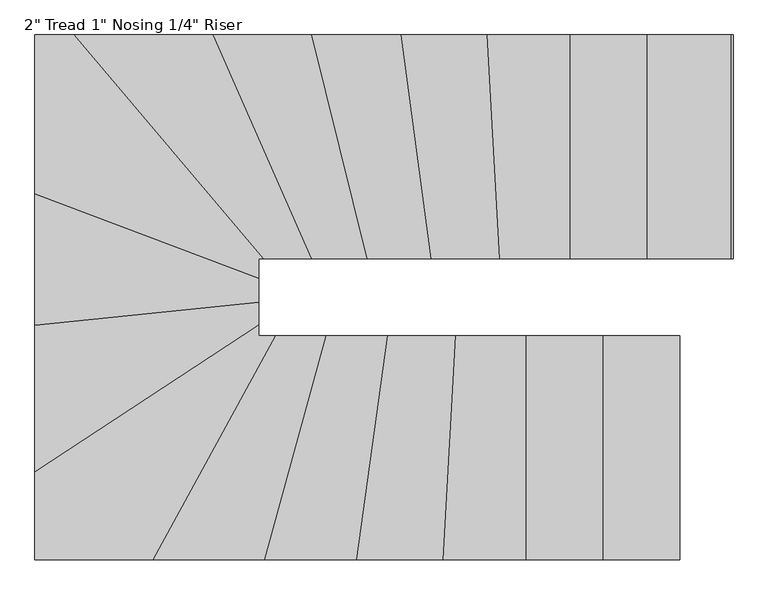
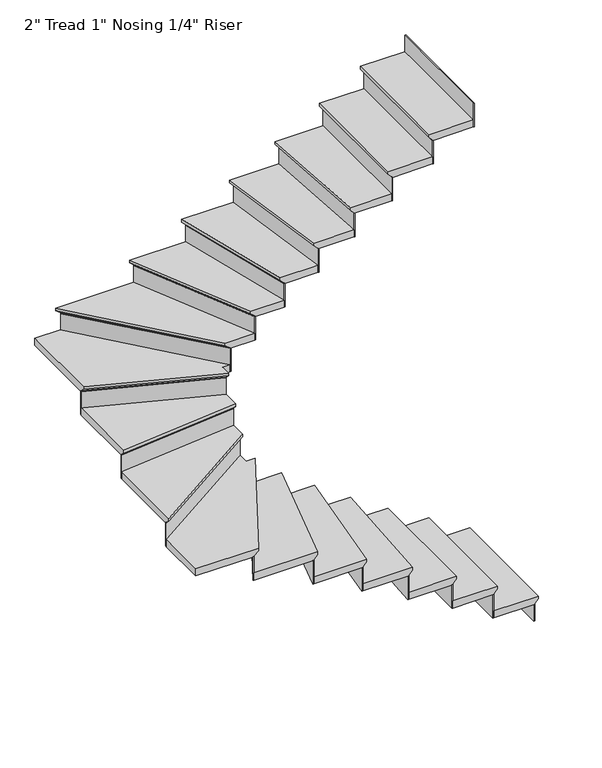
"""IFC4 building model written with IfcOpenShell, lengths in millimetres: stair flight geometry."""

from ifc_helpers import new_model, si_unit, origin, place, context, project, spatial, faceted_brep, source, transform, mapped, element, save


def stair_flight_2a3e21a6(model_context):
    return source(origin(), model_context, "Body", "Brep", [
        faceted_brep([(-12253.9414615, 8989.1162111, 150.2833333), (-12253.9414615, 8989.1162111, 169.3333333), (-12253.9414615, 8176.3162111, 169.3333333), (-12253.9414615, 8176.3162111, 150.2833333), (-12279.3414615, 8989.1162111, 124.8833333), (-12279.3414615, 8176.3162111, 124.8833333), (-12558.7414615, 8989.1162111, 169.3333333), (-12558.7414615, 8176.3162111, 169.3333333), (-12279.3414615, 8176.3162111, 118.5333333), (-12558.7414615, 8176.3162111, 118.5333333), (-12558.7414615, 8989.1162111, 118.5333333), (-12279.3414615, 8989.1162111, 118.5333333)], [[[0, 1, 2, 3]], [[4, 0, 3, 5]], [[2, 1, 6, 7]], [[8, 9, 10, 11]], [[2, 7, 9, 8, 5, 3]], [[8, 11, 4, 5]], [[6, 1, 0, 4, 11, 10]], [[7, 6, 10, 9]]]),
        faceted_brep([(-12279.3414615, 8989.1162111, 118.5333333), (-12279.3414615, 8989.1162111, 0.0), (-12285.6914615, 8989.1162111, 0.0), (-12285.6914615, 8989.1162111, 118.5333333), (-12279.3414615, 8176.3162111, 118.5333333), (-12285.6914615, 8176.3162111, 118.5333333), (-12285.6914615, 8176.3162111, 0.0), (-12279.3414615, 8176.3162111, 0.0)], [[[0, 1, 2, 3]], [[4, 5, 6, 7]], [[1, 0, 4, 7]], [[2, 1, 7, 6]], [[3, 2, 6, 5]], [[0, 3, 5, 4]]]),
        faceted_brep([(-12558.7414615, 8989.1162111, 287.8666667), (-12558.7414615, 8989.1162111, 118.5333333), (-12565.0914615, 8989.1162111, 118.5333333), (-12565.0914615, 8989.1162111, 287.8666667), (-12558.7414615, 8176.3162111, 287.8666667), (-12565.0914615, 8176.3162111, 287.8666667), (-12565.0914615, 8176.3162111, 118.5333333), (-12558.7414615, 8176.3162111, 118.5333333)], [[[0, 1, 2, 3]], [[4, 5, 6, 7]], [[1, 0, 4, 7]], [[2, 1, 7, 6]], [[3, 2, 6, 5]], [[0, 3, 5, 4]]]),
        faceted_brep([(-12533.3414615, 8176.3162111, 338.6666667), (-12533.3414615, 8989.1162111, 338.6666667), (-12838.1414615, 8989.1162111, 338.6666667), (-12838.1414615, 8176.3162111, 338.6666667), (-12558.7414615, 8176.3162111, 287.8666667), (-12838.1414615, 8176.3162111, 287.8666667), (-12838.1414615, 8989.1162111, 287.8666667), (-12558.7414615, 8989.1162111, 287.8666667), (-12558.7414615, 8176.3162111, 294.2166667), (-12533.3414615, 8176.3162111, 319.6166667), (-12558.7414615, 8989.1162111, 294.2166667), (-12533.3414615, 8989.1162111, 319.6166667)], [[[0, 1, 2, 3]], [[4, 5, 6, 7]], [[0, 3, 5, 4, 8, 9]], [[4, 7, 10, 8]], [[2, 1, 11, 10, 7, 6]], [[3, 2, 6, 5]], [[11, 1, 0, 9]], [[10, 11, 9, 8]]]),
        faceted_brep([(-12838.1414615, 8989.1162111, 457.2), (-12838.1414615, 8989.1162111, 287.8666667), (-12844.4914615, 8989.1162111, 287.8666667), (-12844.4914615, 8989.1162111, 457.2), (-12838.1414615, 8176.3162111, 457.2), (-12844.4914615, 8176.3162111, 457.2), (-12844.4914615, 8176.3162111, 287.8666667), (-12838.1414615, 8176.3162111, 287.8666667)], [[[0, 1, 2, 3]], [[4, 5, 6, 7]], [[1, 0, 4, 7]], [[2, 1, 7, 6]], [[3, 2, 6, 5]], [[0, 3, 5, 4]]]),
        faceted_brep([(-12812.7414615, 8176.3162111, 508.0), (-12812.7414615, 8989.1162111, 508.0), (-13095.0084855, 8989.1162111, 508.0), (-13140.152733, 8176.3162111, 508.0), (-12838.1414615, 8176.3162111, 457.2), (-13140.152733, 8176.3162111, 457.2), (-13095.0084855, 8989.1162111, 457.2), (-12838.1414615, 8989.1162111, 457.2), (-12838.1414615, 8176.3162111, 463.55), (-12812.7414615, 8176.3162111, 488.95), (-12838.1414615, 8989.1162111, 463.55), (-12812.7414615, 8989.1162111, 488.95)], [[[0, 1, 2, 3]], [[4, 5, 6, 7]], [[0, 3, 5, 4, 8, 9]], [[4, 7, 10, 8]], [[2, 1, 11, 10, 7, 6]], [[3, 2, 6, 5]], [[11, 1, 0, 9]], [[10, 11, 9, 8]]]),
        faceted_brep([(-13095.0084855, 8989.1162111, 626.5333333), (-13095.0084855, 8989.1162111, 457.2), (-13101.3682724, 8989.1162111, 457.2), (-13101.3682724, 8989.1162111, 626.5333333), (-13140.152733, 8176.3162111, 626.5333333), (-13146.5125199, 8176.3162111, 626.5333333), (-13146.5125199, 8176.3162111, 457.2), (-13140.152733, 8176.3162111, 457.2)], [[[0, 1, 2, 3]], [[4, 5, 6, 7]], [[1, 0, 4, 7]], [[2, 1, 7, 6]], [[3, 2, 6, 5]], [[0, 3, 5, 4]]]),
        faceted_brep([(-13114.7135853, 8176.3162111, 677.3333333), (-13069.5693378, 8989.1162111, 677.3333333), (-13341.0188921, 8989.1162111, 677.3333333), (-13453.3468485, 8176.3162111, 677.3333333), (-13140.152733, 8176.3162111, 626.5333333), (-13453.3468485, 8176.3162111, 626.5333333), (-13341.0188921, 8989.1162111, 626.5333333), (-13095.0084855, 8989.1162111, 626.5333333), (-13140.152733, 8176.3162111, 632.8833333), (-13114.7135853, 8176.3162111, 658.2833333), (-13095.0084855, 8989.1162111, 632.8833333), (-13069.5693378, 8989.1162111, 658.2833333)], [[[0, 1, 2, 3]], [[4, 5, 6, 7]], [[0, 3, 5, 4, 8, 9]], [[4, 7, 10, 8]], [[2, 1, 11, 10, 7, 6]], [[3, 2, 6, 5]], [[11, 1, 0, 9]], [[10, 11, 9, 8]]]),
        faceted_brep([(-13341.0188921, 8989.1162111, 795.8666667), (-13341.0188921, 8989.1162111, 626.5333333), (-13347.4292443, 8989.1162111, 626.5333333), (-13347.4292443, 8989.1162111, 795.8666667), (-13453.3468485, 8176.3162111, 795.8666667), (-13459.7572007, 8176.3162111, 795.8666667), (-13459.7572007, 8176.3162111, 626.5333333), (-13453.3468485, 8176.3162111, 626.5333333)], [[[0, 1, 2, 3]], [[4, 5, 6, 7]], [[1, 0, 4, 7]], [[2, 1, 7, 6]], [[3, 2, 6, 5]], [[0, 3, 5, 4]]]),
        faceted_brep([(-13427.7054397, 8176.3162111, 846.6666667), (-13315.3774833, 8989.1162111, 846.6666667), (-13565.828015, 8989.1162111, 846.6666667), (-13788.7305586, 8176.3162111, 846.6666667), (-13453.3468485, 8176.3162111, 795.8666667), (-13788.7305586, 8176.3162111, 795.8666667), (-13565.828015, 8989.1162111, 795.8666667), (-13341.0188921, 8989.1162111, 795.8666667), (-13453.3468485, 8176.3162111, 802.2166667), (-13427.7054397, 8176.3162111, 827.6166667), (-13341.0188921, 8989.1162111, 802.2166667), (-13315.3774833, 8989.1162111, 827.6166667)], [[[0, 1, 2, 3]], [[4, 5, 6, 7]], [[0, 3, 5, 4, 8, 9]], [[4, 7, 10, 8]], [[2, 1, 11, 10, 7, 6]], [[3, 2, 6, 5]], [[11, 1, 0, 9]], [[10, 11, 9, 8]]]),
        faceted_brep([(-13565.828015, 8989.1162111, 965.2), (-13565.828015, 8989.1162111, 795.8666667), (-13572.4124713, 8989.1162111, 795.8666667), (-13572.4124713, 8989.1162111, 965.2), (-13788.7305586, 8176.3162111, 965.2), (-13795.3150149, 8176.3162111, 965.2), (-13795.3150149, 8176.3162111, 795.8666667), (-13788.7305586, 8176.3162111, 795.8666667)], [[[0, 1, 2, 3]], [[4, 5, 6, 7]], [[1, 0, 4, 7]], [[2, 1, 7, 6]], [[3, 2, 6, 5]], [[0, 3, 5, 4]]]),
        faceted_brep([(-13762.3927333, 8176.3162111, 1016.0), (-13539.4901897, 8989.1162111, 1016.0), (-13750.8519704, 8989.1162111, 1016.0), (-14195.2006773, 8176.3162111, 1016.0), (-13788.7305586, 8176.3162111, 965.2), (-14195.2006773, 8176.3162111, 965.2), (-13750.8519704, 8989.1162111, 965.2), (-13565.828015, 8989.1162111, 965.2), (-13788.7305586, 8176.3162111, 971.55), (-13762.3927333, 8176.3162111, 996.95), (-13565.828015, 8989.1162111, 971.55), (-13539.4901897, 8989.1162111, 996.95)], [[[0, 1, 2, 3]], [[4, 5, 6, 7]], [[0, 3, 5, 4, 8, 9]], [[4, 7, 10, 8]], [[2, 1, 11, 10, 7, 6]], [[3, 2, 6, 5]], [[11, 1, 0, 9]], [[10, 11, 9, 8]]]),
        faceted_brep([(-13750.8519704, 8989.1162111, 1134.5333333), (-13750.8519704, 8989.1162111, 965.2), (-13758.0889334, 8989.1162111, 965.2), (-13758.0889334, 8989.1162111, 1134.5333333), (-14195.2006773, 8176.3162111, 1134.5333333), (-14202.4376404, 8176.3162111, 1134.5333333), (-14202.4376404, 8176.3162111, 965.2), (-14195.2006773, 8176.3162111, 965.2)], [[[0, 1, 2, 3]], [[4, 5, 6, 7]], [[1, 0, 4, 7]], [[2, 1, 7, 6]], [[3, 2, 6, 5]], [[0, 3, 5, 4]]]),
        faceted_brep([(-14594.4731534, 8526.2265371, 1185.3333333), (-14594.4731534, 8176.3162111, 1185.3333333), (-14166.2528253, 8176.3162111, 1185.3333333), (-13721.9041183, 8989.1162111, 1185.3333333), (-13781.6731534, 8989.1162111, 1185.3333333), (-13781.6731534, 9059.6430441, 1185.3333333), (-14594.4731534, 8176.3162111, 1134.5333333), (-14594.4731534, 8526.2265371, 1134.5333333), (-13781.6731534, 9059.6430441, 1134.5333333), (-13781.6731534, 8989.1162111, 1134.5333333), (-13750.8519704, 8989.1162111, 1134.5333333), (-14195.2006773, 8176.3162111, 1134.5333333), (-14195.2006773, 8176.3162111, 1140.8833333), (-14166.2528253, 8176.3162111, 1166.2833333), (-13750.8519704, 8989.1162111, 1140.8833333), (-13721.9041183, 8989.1162111, 1166.2833333)], [[[0, 1, 2, 3, 4, 5]], [[6, 7, 8, 9, 10, 11]], [[1, 0, 7, 6]], [[2, 1, 6, 11, 12, 13]], [[11, 10, 14, 12]], [[4, 3, 15, 14, 10, 9]], [[5, 4, 9, 8]], [[0, 5, 8, 7]], [[15, 3, 2, 13]], [[14, 15, 13, 12]]]),
        faceted_brep([(-13781.6731534, 9059.6430441, 1303.8666667), (-13781.6731534, 9059.6430441, 1134.5333333), (-13781.6731534, 9067.2383734, 1134.5333333), (-13781.6731534, 9067.2383734, 1303.8666667), (-14594.4731534, 8526.2265371, 1303.8666667), (-14594.4731534, 8533.8218664, 1303.8666667), (-14594.4731534, 8533.8218664, 1134.5333333), (-14594.4731534, 8526.2265371, 1134.5333333)], [[[0, 1, 2, 3]], [[4, 5, 6, 7]], [[1, 0, 4, 7]], [[2, 1, 7, 6]], [[3, 2, 6, 5]], [[0, 3, 5, 4]]]),
        faceted_brep([(-14594.4731534, 8495.8452201, 1354.6666667), (-13781.6731534, 9029.2617271, 1354.6666667), (-13781.6731534, 9137.1899259, 1354.6666667), (-14594.4731534, 9053.7994193, 1354.6666667), (-14594.4731534, 8526.2265371, 1303.8666667), (-14594.4731534, 9053.7994193, 1303.8666667), (-13781.6731534, 9137.1899259, 1303.8666667), (-13781.6731534, 9059.6430441, 1303.8666667), (-14594.4731534, 8526.2265371, 1310.2166667), (-14594.4731534, 8495.8452201, 1335.6166667), (-13781.6731534, 9059.6430441, 1310.2166667), (-13781.6731534, 9029.2617271, 1335.6166667)], [[[0, 1, 2, 3]], [[4, 5, 6, 7]], [[0, 3, 5, 4, 8, 9]], [[4, 7, 10, 8]], [[3, 2, 6, 5]], [[11, 1, 0, 9]], [[10, 11, 9, 8]], [[2, 1, 11, 10, 7, 6]]]),
        faceted_brep([(-13781.6731534, 9137.1899259, 1473.2), (-13781.6731534, 9137.1899259, 1303.8666667), (-13781.6731534, 9143.5732587, 1303.8666667), (-13781.6731534, 9143.5732587, 1473.2), (-14594.4731534, 9053.7994193, 1473.2), (-14594.4731534, 9060.182752, 1473.2), (-14594.4731534, 9060.182752, 1303.8666667), (-14594.4731534, 9053.7994193, 1303.8666667)], [[[0, 1, 2, 3]], [[4, 5, 6, 7]], [[1, 0, 4, 7]], [[2, 1, 7, 6]], [[3, 2, 6, 5]], [[0, 3, 5, 4]]]),
        faceted_brep([(-14594.4731534, 9028.2660883, 1524.0), (-13781.6731534, 9111.6565949, 1524.0), (-13781.6731534, 9225.8746832, 1524.0), (-14594.4731534, 9533.0408462, 1524.0), (-14594.4731534, 9053.7994193, 1473.2), (-14594.4731534, 9533.0408462, 1473.2), (-13781.6731534, 9225.8746832, 1473.2), (-13781.6731534, 9137.1899259, 1473.2), (-14594.4731534, 9053.7994193, 1479.55), (-14594.4731534, 9028.2660883, 1504.95), (-13781.6731534, 9137.1899259, 1479.55), (-13781.6731534, 9111.6565949, 1504.95)], [[[0, 1, 2, 3]], [[4, 5, 6, 7]], [[0, 3, 5, 4, 8, 9]], [[4, 7, 10, 8]], [[2, 1, 11, 10, 7, 6]], [[3, 2, 6, 5]], [[11, 1, 0, 9]], [[10, 11, 9, 8]]]),
        faceted_brep([(-13781.6731534, 9225.8746832, 1642.5333333), (-13781.6731534, 9225.8746832, 1473.2), (-13781.6731534, 9232.662999, 1473.2), (-13781.6731534, 9232.662999, 1642.5333333), (-14594.4731534, 9533.0408462, 1642.5333333), (-14594.4731534, 9539.829162, 1642.5333333), (-14594.4731534, 9539.829162, 1473.2), (-14594.4731534, 9533.0408462, 1473.2)], [[[0, 1, 2, 3]], [[4, 5, 6, 7]], [[1, 0, 4, 7]], [[2, 1, 7, 6]], [[3, 2, 6, 5]], [[0, 3, 5, 4]]]),
        faceted_brep([(-14418.4386981, 10081.3162111, 1693.3333333), (-14594.4731534, 10081.3162111, 1693.3333333), (-14594.4731534, 9505.8875831, 1693.3333333), (-13781.6731534, 9198.7214201, 1693.3333333), (-13781.6731534, 9268.5162111, 1693.3333333), (-13730.7180609, 9268.5162111, 1693.3333333), (-14594.4731534, 10081.3162111, 1642.5333333), (-14418.4386981, 10081.3162111, 1642.5333333), (-13730.7180609, 9268.5162111, 1642.5333333), (-13781.6731534, 9268.5162111, 1642.5333333), (-13781.6731534, 9225.8746832, 1642.5333333), (-14594.4731534, 9533.0408462, 1642.5333333), (-13781.6731534, 9225.8746832, 1648.8833333), (-14594.4731534, 9533.0408462, 1648.8833333), (-13781.6731534, 9198.7214201, 1674.2833333), (-14594.4731534, 9505.8875831, 1674.2833333)], [[[0, 1, 2, 3, 4, 5]], [[6, 7, 8, 9, 10, 11]], [[1, 0, 7, 6]], [[11, 10, 12, 13]], [[4, 3, 14, 12, 10, 9]], [[5, 4, 9, 8]], [[0, 5, 8, 7]], [[14, 3, 2, 15]], [[12, 14, 15, 13]], [[2, 1, 6, 11, 13, 15]]]),
        faceted_brep([(-13730.7180609, 9268.5162111, 1811.8666667), (-13730.7180609, 9268.5162111, 1642.5333333), (-13722.4000282, 9268.5162111, 1642.5333333), (-13722.4000282, 9268.5162111, 1811.8666667), (-14418.4386981, 10081.3162111, 1811.8666667), (-14410.1206654, 10081.3162111, 1811.8666667), (-14410.1206654, 10081.3162111, 1642.5333333), (-14418.4386981, 10081.3162111, 1642.5333333)], [[[0, 1, 2, 3]], [[4, 5, 6, 7]], [[1, 0, 4, 7]], [[2, 1, 7, 6]], [[3, 2, 6, 5]], [[0, 3, 5, 4]]]),
        faceted_brep([(-14451.7108288, 10081.3162111, 1862.6666667), (-13763.9901916, 9268.5162111, 1862.6666667), (-13561.8866362, 9268.5162111, 1862.6666667), (-13919.4471597, 10081.3162111, 1862.6666667), (-14418.4386981, 10081.3162111, 1811.8666667), (-13919.4471597, 10081.3162111, 1811.8666667), (-13561.8866362, 9268.5162111, 1811.8666667), (-13730.7180609, 9268.5162111, 1811.8666667), (-14418.4386981, 10081.3162111, 1818.2166667), (-14451.7108288, 10081.3162111, 1843.6166667), (-13730.7180609, 9268.5162111, 1818.2166667), (-13763.9901916, 9268.5162111, 1843.6166667)], [[[0, 1, 2, 3]], [[4, 5, 6, 7]], [[0, 3, 5, 4, 8, 9]], [[4, 7, 10, 8]], [[2, 1, 11, 10, 7, 6]], [[3, 2, 6, 5]], [[11, 1, 0, 9]], [[10, 11, 9, 8]]]),
        faceted_brep([(-13561.8866362, 9268.5162111, 1981.2), (-13561.8866362, 9268.5162111, 1811.8666667), (-13554.9493589, 9268.5162111, 1811.8666667), (-13554.9493589, 9268.5162111, 1981.2), (-13919.4471597, 10081.3162111, 1981.2), (-13912.5098824, 10081.3162111, 1981.2), (-13912.5098824, 10081.3162111, 1811.8666667), (-13919.4471597, 10081.3162111, 1811.8666667)], [[[0, 1, 2, 3]], [[4, 5, 6, 7]], [[1, 0, 4, 7]], [[2, 1, 7, 6]], [[3, 2, 6, 5]], [[0, 3, 5, 4]]]),
        faceted_brep([(-13947.1962688, 10081.3162111, 2032.0), (-13589.6357452, 9268.5162111, 2032.0), (-13361.4241214, 9268.5162111, 2032.0), (-13564.2501156, 10081.3162111, 2032.0), (-13919.4471597, 10081.3162111, 1981.2), (-13564.2501156, 10081.3162111, 1981.2), (-13361.4241214, 9268.5162111, 1981.2), (-13561.8866362, 9268.5162111, 1981.2), (-13919.4471597, 10081.3162111, 1987.55), (-13947.1962688, 10081.3162111, 2012.95), (-13561.8866362, 9268.5162111, 1987.55), (-13589.6357452, 9268.5162111, 2012.95)], [[[0, 1, 2, 3]], [[4, 5, 6, 7]], [[0, 3, 5, 4, 8, 9]], [[4, 7, 10, 8]], [[2, 1, 11, 10, 7, 6]], [[3, 2, 6, 5]], [[11, 1, 0, 9]], [[10, 11, 9, 8]]]),
        faceted_brep([(-13361.4241214, 9268.5162111, 2150.5333333), (-13361.4241214, 9268.5162111, 1981.2), (-13354.8793993, 9268.5162111, 1981.2), (-13354.8793993, 9268.5162111, 2150.5333333), (-13564.2501156, 10081.3162111, 2150.5333333), (-13557.7053934, 10081.3162111, 2150.5333333), (-13557.7053934, 10081.3162111, 1981.2), (-13564.2501156, 10081.3162111, 1981.2)], [[[0, 1, 2, 3]], [[4, 5, 6, 7]], [[1, 0, 4, 7]], [[2, 1, 7, 6]], [[3, 2, 6, 5]], [[0, 3, 5, 4]]]),
        faceted_brep([(-13590.4290041, 10081.3162111, 2201.3333333), (-13387.6030099, 9268.5162111, 2201.3333333), (-13129.6274374, 9268.5162111, 2201.3333333), (-13238.3521036, 10081.3162111, 2201.3333333), (-13564.2501156, 10081.3162111, 2150.5333333), (-13238.3521036, 10081.3162111, 2150.5333333), (-13129.6274374, 9268.5162111, 2150.5333333), (-13361.4241214, 9268.5162111, 2150.5333333), (-13564.2501156, 10081.3162111, 2156.8833333), (-13590.4290041, 10081.3162111, 2182.2833333), (-13361.4241214, 9268.5162111, 2156.8833333), (-13387.6030099, 9268.5162111, 2182.2833333)], [[[0, 1, 2, 3]], [[4, 5, 6, 7]], [[0, 3, 5, 4, 8, 9]], [[4, 7, 10, 8]], [[2, 1, 11, 10, 7, 6]], [[3, 2, 6, 5]], [[11, 1, 0, 9]], [[10, 11, 9, 8]]]),
        faceted_brep([(-13129.6274374, 9268.5162111, 2319.8666667), (-13129.6274374, 9268.5162111, 2150.5333333), (-13123.2208783, 9268.5162111, 2150.5333333), (-13123.2208783, 9268.5162111, 2319.8666667), (-13238.3521036, 10081.3162111, 2319.8666667), (-13231.9455444, 10081.3162111, 2319.8666667), (-13231.9455444, 10081.3162111, 2150.5333333), (-13238.3521036, 10081.3162111, 2150.5333333)], [[[0, 1, 2, 3]], [[4, 5, 6, 7]], [[1, 0, 4, 7]], [[2, 1, 7, 6]], [[3, 2, 6, 5]], [[0, 3, 5, 4]]]),
        faceted_brep([(-13263.9783401, 10081.3162111, 2370.6666667), (-13155.2536739, 9268.5162111, 2370.6666667), (-12882.0481928, 9268.5162111, 2370.6666667), (-12927.5044406, 10081.3162111, 2370.6666667), (-13238.3521036, 10081.3162111, 2319.8666667), (-12927.5044406, 10081.3162111, 2319.8666667), (-12882.0481928, 9268.5162111, 2319.8666667), (-13129.6274374, 9268.5162111, 2319.8666667), (-13238.3521036, 10081.3162111, 2326.2166667), (-13263.9783401, 10081.3162111, 2351.6166667), (-13129.6274374, 9268.5162111, 2326.2166667), (-13155.2536739, 9268.5162111, 2351.6166667)], [[[0, 1, 2, 3]], [[4, 5, 6, 7]], [[0, 3, 5, 4, 8, 9]], [[4, 7, 10, 8]], [[2, 1, 11, 10, 7, 6]], [[3, 2, 6, 5]], [[11, 1, 0, 9]], [[10, 11, 9, 8]]]),
        faceted_brep([(-12882.0481928, 9268.5162111, 2489.2), (-12882.0481928, 9268.5162111, 2319.8666667), (-12875.6882702, 9268.5162111, 2319.8666667), (-12875.6882702, 9268.5162111, 2489.2), (-12927.5044406, 10081.3162111, 2489.2), (-12921.144518, 10081.3162111, 2489.2), (-12921.144518, 10081.3162111, 2319.8666667), (-12927.5044406, 10081.3162111, 2319.8666667)], [[[0, 1, 2, 3]], [[4, 5, 6, 7]], [[1, 0, 4, 7]], [[2, 1, 7, 6]], [[3, 2, 6, 5]], [[0, 3, 5, 4]]]),
        faceted_brep([(-12952.9441309, 10081.3162111, 2540.0), (-12907.4878831, 9268.5162111, 2540.0), (-12625.416007, 9268.5162111, 2540.0), (-12625.416007, 10081.3162111, 2540.0), (-12927.5044406, 10081.3162111, 2489.2), (-12625.416007, 10081.3162111, 2489.2), (-12625.416007, 9268.5162111, 2489.2), (-12882.0481928, 9268.5162111, 2489.2), (-12927.5044406, 10081.3162111, 2495.55), (-12952.9441309, 10081.3162111, 2520.95), (-12882.0481928, 9268.5162111, 2495.55), (-12907.4878831, 9268.5162111, 2520.95)], [[[0, 1, 2, 3]], [[4, 5, 6, 7]], [[0, 3, 5, 4, 8, 9]], [[4, 7, 10, 8]], [[2, 1, 11, 10, 7, 6]], [[3, 2, 6, 5]], [[11, 1, 0, 9]], [[10, 11, 9, 8]]]),
        faceted_brep([(-12625.416007, 9268.5162111, 2658.5333333), (-12625.416007, 9268.5162111, 2489.2), (-12619.066007, 9268.5162111, 2489.2), (-12619.066007, 9268.5162111, 2658.5333333), (-12625.416007, 10081.3162111, 2658.5333333), (-12619.066007, 10081.3162111, 2658.5333333), (-12619.066007, 10081.3162111, 2489.2), (-12625.416007, 10081.3162111, 2489.2)], [[[0, 1, 2, 3]], [[4, 5, 6, 7]], [[1, 0, 4, 7]], [[2, 1, 7, 6]], [[3, 2, 6, 5]], [[0, 3, 5, 4]]]),
        faceted_brep([(-12650.816007, 10081.3162111, 2709.3333333), (-12650.816007, 9268.5162111, 2709.3333333), (-12346.016007, 9268.5162111, 2709.3333333), (-12346.016007, 10081.3162111, 2709.3333333), (-12625.416007, 10081.3162111, 2658.5333333), (-12346.016007, 10081.3162111, 2658.5333333), (-12346.016007, 9268.5162111, 2658.5333333), (-12625.416007, 9268.5162111, 2658.5333333), (-12625.416007, 10081.3162111, 2664.8833333), (-12650.816007, 10081.3162111, 2690.2833333), (-12625.416007, 9268.5162111, 2664.8833333), (-12650.816007, 9268.5162111, 2690.2833333)], [[[0, 1, 2, 3]], [[4, 5, 6, 7]], [[0, 3, 5, 4, 8, 9]], [[4, 7, 10, 8]], [[2, 1, 11, 10, 7, 6]], [[3, 2, 6, 5]], [[11, 1, 0, 9]], [[10, 11, 9, 8]]]),
        faceted_brep([(-12346.016007, 9268.5162111, 2827.8666667), (-12346.016007, 9268.5162111, 2658.5333333), (-12339.666007, 9268.5162111, 2658.5333333), (-12339.666007, 9268.5162111, 2827.8666667), (-12346.016007, 10081.3162111, 2827.8666667), (-12339.666007, 10081.3162111, 2827.8666667), (-12339.666007, 10081.3162111, 2658.5333333), (-12346.016007, 10081.3162111, 2658.5333333)], [[[0, 1, 2, 3]], [[4, 5, 6, 7]], [[1, 0, 4, 7]], [[2, 1, 7, 6]], [[3, 2, 6, 5]], [[0, 3, 5, 4]]]),
        faceted_brep([(-12066.616007, 9268.5162111, 2997.2), (-12066.616007, 9268.5162111, 2827.8666667), (-12060.266007, 9268.5162111, 2827.8666667), (-12060.266007, 9268.5162111, 2997.2), (-12066.616007, 10081.3162111, 2997.2), (-12060.266007, 10081.3162111, 2997.2), (-12060.266007, 10081.3162111, 2827.8666667), (-12066.616007, 10081.3162111, 2827.8666667)], [[[0, 1, 2, 3]], [[4, 5, 6, 7]], [[1, 0, 4, 7]], [[2, 1, 7, 6]], [[3, 2, 6, 5]], [[0, 3, 5, 4]]]),
        faceted_brep([(-12371.416007, 10081.3162111, 2878.6666667), (-12371.416007, 9268.5162111, 2878.6666667), (-12066.616007, 9268.5162111, 2878.6666667), (-12066.616007, 10081.3162111, 2878.6666667), (-12346.016007, 10081.3162111, 2827.8666667), (-12066.616007, 10081.3162111, 2827.8666667), (-12066.616007, 9268.5162111, 2827.8666667), (-12346.016007, 9268.5162111, 2827.8666667), (-12346.016007, 10081.3162111, 2834.2166667), (-12371.416007, 10081.3162111, 2859.6166667), (-12346.016007, 9268.5162111, 2834.2166667), (-12371.416007, 9268.5162111, 2859.6166667)], [[[0, 1, 2, 3]], [[4, 5, 6, 7]], [[0, 3, 5, 4, 8, 9]], [[4, 7, 10, 8]], [[2, 1, 11, 10, 7, 6]], [[3, 2, 6, 5]], [[11, 1, 0, 9]], [[10, 11, 9, 8]]]),
    ])


if __name__ == "__main__":
    model = new_model("IFC4")
    model_context = context("Model", 3, world=origin())
    ifc_project = project(units=[si_unit("LENGTHUNIT", "METRE", prefix="MILLI")], contexts=[model_context])
    site = spatial("IfcSite", under=ifc_project)
    building = spatial("IfcBuilding", under=site)
    placement = place(None, origin())
    stair_flight_shape = stair_flight_2a3e21a6(model_context)
    element("IfcStairFlight", 1, ObjectType="2\" Tread 1\" Nosing 1/4\" Riser", at=placement, inside=building, context=model_context, shape_type="MappedRepresentation", body=[
        mapped(stair_flight_shape, transform((0.0, 0.0, 0.0), x_axis=(1.0, 0.0, 0.0), y_axis=(0.0, 1.0, 0.0), z_axis=(0.0, 0.0, 1.0))),
    ])
    save(model, "model.ifc")
